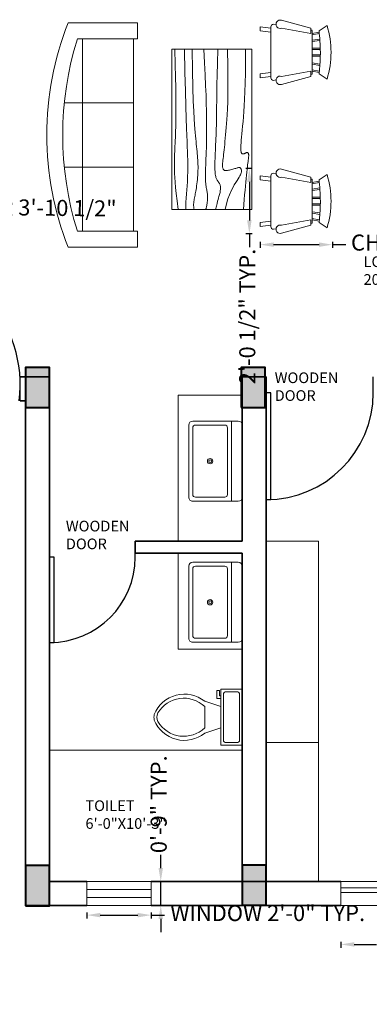
# Model space of a CAD drawing. Units: inches. Extents: x 2845 to 3575, y 808 to 1996.
# Tile 3 of 6: x 3173 to 3304, y 1215 to 1584. Entities that reach past the tile are written whole.
import ezdxf

# ---------------------------------------------------------------- set-up
doc = ezdxf.new("R2010")
doc.units = ezdxf.units.IN
for name, color, linetype, lineweight in [('A-ANNO-DIMS', 2, 'Continuous', 18), ('A-ANNO-TEXT', 7, 'Continuous', 18), ('A-AREA-IDEN', 7, 'Continuous', 18), ('A-COLS', 7, 'Continuous', 40), ('A-DOOR', 34, 'Continuous', 25), ('A-FLOR-CASE', 30, 'Continuous', 18), ('A-FLOR-FIXT', 8, 'Continuous', 18), ('A-FURN', 30, 'Continuous', 18), ('A-GLAZ', 4, 'Continuous', 18), ('A-WALL', 1, 'Continuous', 35)]:
    doc.layers.add(name, color=color, linetype=linetype, lineweight=lineweight)
doc.styles.get("Standard").update_dxf_attribs({"font": 'arial.ttf'})
doc.dimstyles.new('ISO-25', dxfattribs={"dimtxt": 6, "dimasz": 5, "dimexe": 1.25, "dimexo": 0.625, "dimtad": 0, "dimlunit": 4, "dimtxsty": 'Standard', "dimcen": 2.5, "dimclrd": 1, "dimclre": 1, "dimclrt": 1, "dimadec": 0, "dimazin": 0, "dimtfac": 1, "dimtmove": 0, "dimatfit": 3, "dimfxl": 1, "dimfxlon": 1, "dimfrac": 1, "dimarcsym": 0})

# ---------------------------------------------------------------- blocks, each defined once
blk = doc.blocks.new('*U4')
for p, q in [((0, 0), (0, 6)), ((32, 0), (32, 6))]:
    blk.add_line(p, q)
blk.add_lwpolyline([(0, 0), (0, -32), (1.75, -32), (1.75, 0)], close=True)
blk.add_arc((0, 0), 32, 270, 0)
blk = doc.blocks.new('*U5')
for p, q in [((0, 0), (0, 6)), ((40, 0), (40, 6))]:
    blk.add_line(p, q)
blk.add_lwpolyline([(0, 0), (0, -40), (1.75, -40), (1.75, 0)], close=True)
blk.add_arc((0, 0), 40, 270, 0)
blk = doc.blocks.new('Sofa - Roundback 7 ft.')
for p, q in [((-12.00002, -32.4421), (-12.00003, -6.5971)), ((11.99997, -32.4421), (11.99998, -6.5971)), ((-36.000027, -34), (-36.000027, -11.4696)), ((-35.999844, -13.3819), (35.9998, -13.3819)), ((35.99998, -34), (35.99998, -11.4696)), ((-36.000027, -32.4421), (35.99998, -32.4421))]:
    blk.add_line(p, q)
for points in [[(-36.000027, -34), (-42.000027, -34), (-42.000027, -8)], [(41.99998, -8), (41.99998, -34), (35.99998, -34)]]:
    blk.add_lwpolyline(points)
for centre, radius, start, end in [((0, -114.25), 114.25, 68.43141, 111.5686), ((-0.00001, -127.1968), 121.1968, 72.72033, 107.2797)]:
    blk.add_arc(centre, radius, start, end)
blk = doc.blocks.new('Chair - Rocking')
for p, q in [((-8, -4.5), (-10, -1.5)), ((8, -4.5), (10, -1.5)), ((-8.23428, -6.99939), (-8.3093, -7.47958)), ((-8.23041, -7), (8.23915, -7)), ((-7.5, -4.5), (-7, -7)), ((-6.5, -7), (-7.02225, -4.43)), ((-4.5, -7), (-4.96674, -4.19951)), ((-4, -7), (-4.40532, -4.16272)), ((-1.5, -4.05012), (-1.5, -7)), ((-1, -7), (-1, -4.05012)), ((1, -7), (1, -4.04655)), ((1.5, -4.05012), (1.5, -7)), ((4, -7), (4.40187, -4.18694)), ((4.5, -7), (4.96761, -4.19437)), ((6.5, -7), (7, -4.4057)), ((7.5, -4.5), (7, -7)), ((8.31071, -7.48854), (8.23449, -7.00073)), ((-9, -7.5), (-12, -18.49999)), ((-7, -7.5), (-9, -7.5)), ((-9, -18.49999), (-7, -7.5)), ((7, -7.5), (9, -7.5)), ((9, -18.49999), (7, -7.5)), ((9, -7.5), (12, -18.49999)), ((-10.36644, -20.64523), (-10.5, -21.49999)), ((10.5, -21.49999), (10.3575, -20.58798)), ((-9, -22.49999), (-9.5, -26.49999)), ((0, -22.49999), (-9.5, -22.49999)), ((-8, -26.49999), (-7.5, -22.49999)), ((0, -22.49999), (9.5, -22.49999)), ((8, -26.49999), (7.5, -22.49999)), ((9, -22.49999), (9.5, -26.49999)), ((-9.5, -26.49999), (-8, -26.49999)), ((9.5, -26.49999), (8, -26.49999))]:
    blk.add_line(p, q)
for centre, radius, start, end in [((0, -34.08333), 34.08333, 72.93847, 107.0615), ((0, -68.25004), 64.25, 93.92211, 97.15267), ((0, -68.25004), 64.25, 82.84733, 93.92211), ((-10.5, -18.99999), 1.58114, 161.5651, 18.43495), ((-9.5, -21.49999), 1, 180, 270), ((10.5, -18.99999), 1.58114, 161.5651, 18.43495), ((9.5, -21.49999), 1, 270, 0)]:
    blk.add_arc(centre, radius, start, end)
blk = doc.blocks.new('Sink-single - 30 in top')
blk.add_line((-15, -3.999996), (15, -3.999996))
for points in [[(-13.5, 0), (13.5, 0)], [(-15, -18.499996), (-15, -1.5)], [(15, -1.5), (15, -18.499996)], [(-13.5, -17.499996), (-13.5, -6.499996)], [(-12.5, -5.499996), (12.5, -5.499996)], [(13.5, -6.499996), (13.5, -17.499996)], [(13.5, -19.999996), (-13.5, -19.999996)], [(12.5, -18.499996), (-12.5, -18.499996)]]:
    blk.add_lwpolyline(points)
for radius in [1, 0.5]:
    blk.add_circle((0, -11.999996), radius)
for centre, radius, start, end in [((-13.5, -1.5), 1.5, 90, 180), ((13.5, -1.5), 1.5, 0, 90), ((-12.5, -6.499996), 1, 90, 180), ((12.5, -6.499996), 1, 0, 90), ((-12.5, -17.499996), 1, 180, 270), ((12.5, -17.499996), 1, 270, 0), ((-13.5, -18.499996), 1.5, 180, 270), ((13.5, -18.499996), 1.5, 270, 0)]:
    blk.add_arc(centre, radius, start, end)
blk = doc.blocks.new('Toilet - top')
for p, q in [((9.5, -6), (9.5, -2)), ((-10, -8.5), (-8, -8.5)), ((-10, -9.5), (-10, -8.5)), ((-7, -9.5), (-10, -9.5)), ((-8, -8.5), (-8, -8)), ((-7, -8), (-7, -9.5)), ((-4, -8), (-6, -14)), ((4, -8), (6, -14)), ((4, -14), (-4, -14))]:
    blk.add_line(p, q)
blk.add_lwpolyline([(10.5, -8), (10.5, 0), (-10.5, 0), (-10.5, -8)], close=True)
for points in [[(-9.5, -2), (-9.5, -6)], [(8.5, -1), (-8.5, -1)], [(-8.5, -7), (8.5, -7)]]:
    blk.add_lwpolyline(points)
for centre, radius, start, end in [((-8.62, -1.88), 0.884, 81.8699, 188.1301), ((8.62, -1.88), 0.884, 351.8699, 98.1301), ((-8.62, -6.12), 0.884, 171.8699, 278.1301), ((8.62, -6.12), 0.884, 261.8699, 8.1301), ((3.52, -21.58), 12.17, 141.4691, 247.9714), ((4.2, -21.82), 11.33, 136.3677, 238.9468), ((-3.52, -21.58), 12.17, 292.0284, 38.5307), ((-4.2, -21.82), 11.33, 301.053, 43.6321), ((0, -27.88), 4, 245.7318, 294.2682), ((0, -29), 4, 254.8605, 285.1395)]:
    blk.add_arc(centre, radius, start, end)
blk = doc.blocks.new('Table - Rectangular Woodgrain 60 x 30 in.')
for p, q in [((0, 0), (0, -30)), ((60, 0), (0, 0)), ((60, -30), (60, 0)), ((0, -30), (60, -30))]:
    blk.add_line(p, q)
for points in [[(0, -2.4), (4.8155, -2.418), (9.0302, -2.4688), (12.709, -2.5477), (15.9167, -2.65), (18.7181, -2.7711), (21.1781, -2.9063), (23.3616, -3.0508), (25.3333, -3.2), (27.1477, -3.3495), (28.8172, -3.4958), (30.3437, -3.636), (31.7291, -3.7667), (32.9756, -3.8849), (34.0849, -3.9875), (35.059, -4.0714), (35.9, -4.1334), (36.6114, -4.1711), (37.2041, -4.1854), (37.6906, -4.1779), (38.0833, -4.15), (38.3948, -4.1034), (38.6375, -4.0396), (38.8239, -3.9602), (38.9666, -3.8667), (39.0764, -3.7608), (39.1573, -3.6448), (39.2116, -3.521), (39.2416, -3.3917), (39.2498, -3.2593), (39.2385, -3.1261), (39.21, -2.9944), (39.1666, -2.8667), (39.111, -2.7447), (39.0468, -2.6281), (38.978, -2.5163), (38.9083, -2.4083), (38.8418, -2.3035), (38.7823, -2.201), (38.7337, -2.1001), (38.7, -2), (38.6844, -1.9003), (38.6875, -1.8021), (38.7094, -1.707), (38.75, -1.6167), (38.8094, -1.5326), (38.8875, -1.4563), (38.9844, -1.3893), (39.1, -1.3333), (39.2351, -1.2896), (39.3937, -1.2583), (39.5804, -1.2396), (39.8, -1.2333), (40.057, -1.2396), (40.3562, -1.2583), (40.7023, -1.2896), (41.1, -1.3333), (41.5547, -1.3895), (42.0755, -1.4573), (42.6721, -1.5361), (43.3542, -1.625), (44.1316, -1.7233), (45.014, -1.8302), (46.0114, -1.9449), (47.1333, -2.0667), (48.3862, -2.1947), (49.7625, -2.3281), (51.2513, -2.4663), (52.8416, -2.6083), (54.5226, -2.7535), (56.2833, -2.9011), (58.1127, -3.0501), (60, -3.2)], [(0, -9.2), (6.5759, -9.0858), (11.9385, -9.0365), (16.2527, -9.0418), (19.6833, -9.0917), (22.3952, -9.1759), (24.5531, -9.2844), (26.322, -9.4069), (27.8666, -9.5333), (29.3241, -9.6553), (30.7203, -9.7719), (32.0532, -9.8837), (33.3208, -9.9917), (34.5213, -10.0965), (35.6526, -10.199), (36.7128, -10.2999), (37.7, -10.4), (38.6129, -10.4996), (39.4531, -10.5969), (40.223, -10.6895), (40.925, -10.775), (41.5613, -10.8512), (42.1344, -10.9156), (42.6465, -10.966), (43.1, -11), (43.4976, -11.0158), (43.8437, -11.0136), (44.143, -10.9942), (44.4, -10.9583), (44.6195, -10.9069), (44.8062, -10.8406), (44.9648, -10.7603), (45.1, -10.6667), (45.2155, -10.5598), (45.3114, -10.4365), (45.3871, -10.2929), (45.4416, -10.125), (45.4743, -9.929), (45.4844, -9.7011), (45.4709, -9.4371), (45.4333, -9.1333), (45.3716, -8.7883), (45.2896, -8.4104), (45.1919, -8.0107), (45.0833, -7.6), (44.9685, -7.1893), (44.8521, -6.7896), (44.7388, -6.4117), (44.6333, -6.0667), (44.54, -5.7628), (44.4614, -5.4979), (44.4001, -5.2675), (44.3583, -5.0667), (44.3384, -4.8909), (44.3427, -4.7354), (44.3736, -4.5956), (44.4333, -4.4667), (44.5236, -4.3453), (44.6427, -4.2333), (44.7884, -4.1339), (44.9583, -4.05), (45.1501, -3.9849), (45.3614, -3.9417), (45.59, -3.9234), (45.8333, -3.9333), (46.0915, -3.9749), (46.3734, -4.0531), (46.6906, -4.1736), (47.0542, -4.3417), (47.4756, -4.5629), (47.9661, -4.8427), (48.5372, -5.1866), (49.2, -5.6), (49.9676, -6.0844), (50.8594, -6.625), (51.8965, -7.2031), (53.1, -7.8), (54.491, -8.3969), (56.0906, -8.975), (57.9199, -9.5156), (60, -10)], [(0, -12.8), (5.1847, -12.9322), (9.6213, -13.0323), (13.3963, -13.1059), (16.5958, -13.1583), (19.3063, -13.1952), (21.614, -13.2219), (23.6054, -13.2439), (25.3666, -13.2667), (26.9728, -13.2947), (28.4531, -13.3281), (29.8256, -13.3663), (31.1083, -13.4083), (32.3191, -13.4535), (33.476, -13.501), (34.597, -13.5501), (35.7, -13.6), (36.7984, -13.6497), (37.8875, -13.6979), (38.9578, -13.743), (40, -13.7833), (41.0047, -13.8174), (41.9625, -13.8438), (42.864, -13.8607), (43.7, -13.8667), (44.4631, -13.8604), (45.1552, -13.8417), (45.7801, -13.8104), (46.3416, -13.7667), (46.8439, -13.7104), (47.2906, -13.6417), (47.6858, -13.5604), (48.0333, -13.4667), (48.3375, -13.3608), (48.6042, -13.2448), (48.8396, -13.121), (49.05, -12.9917), (49.2417, -12.8593), (49.4208, -12.7261), (49.5937, -12.5944), (49.7667, -12.4667), (49.9452, -12.3451), (50.1323, -12.2313), (50.3303, -12.1268), (50.5416, -12.0333), (50.7686, -11.9524), (51.0135, -11.8854), (51.2788, -11.8341), (51.5666, -11.8), (51.8785, -11.7843), (52.2116, -11.7865), (52.562, -11.8059), (52.926, -11.8417), (53.2998, -11.8931), (53.6795, -11.9594), (54.0614, -12.0397), (54.4416, -12.1333), (54.8223, -12.2401), (55.2293, -12.3625), (55.6942, -12.5037), (56.2489, -12.6667), (56.9251, -12.8547), (57.7545, -13.0708), (58.7689, -13.3182), (60, -13.6)], [(0, -18), (5.124, -17.7273), (9.6609, -17.5057), (13.6705, -17.3303), (17.2125, -17.1958), (20.3467, -17.0973), (23.1328, -17.0297), (25.6307, -16.9878), (27.9, -16.9667), (29.9928, -16.9617), (31.9302, -16.9703), (33.7254, -16.9907), (35.3917, -17.0208), (36.9423, -17.0588), (38.3906, -17.1026), (39.7499, -17.1503), (41.0333, -17.2), (42.2519, -17.2496), (43.4073, -17.2969), (44.4986, -17.3395), (45.525, -17.375), (46.4858, -17.4012), (47.3802, -17.4156), (48.2074, -17.416), (48.9667, -17.4), (49.6583, -17.3662), (50.2872, -17.3167), (50.8595, -17.2547), (51.3812, -17.1833), (51.8584, -17.1057), (52.2971, -17.025), (52.7034, -16.9443), (53.0833, -16.8667), (53.443, -16.7951), (53.789, -16.7313), (54.128, -16.6768), (54.4666, -16.6334), (54.8115, -16.6024), (55.1693, -16.5854), (55.5465, -16.5841), (55.95, -16.6), (56.3828, -16.6337), (56.8346, -16.6823), (57.2915, -16.7418), (57.7396, -16.8084), (58.165, -16.878), (58.5539, -16.9469), (58.8924, -17.0111), (59.1666, -17.0667), (59.3679, -17.1107), (59.5078, -17.1438), (59.6032, -17.1675), (59.6708, -17.1833), (59.7275, -17.193), (59.7901, -17.1979), (59.8753, -17.1998), (60, -17.2)], [(0, -22.4), (8.0098, -22.2501), (14.4094, -22.1011), (19.4168, -21.9535), (23.25, -21.8083), (26.1269, -21.6663), (28.2656, -21.5281), (29.884, -21.3947), (31.2, -21.2667), (32.3967, -21.1448), (33.5172, -21.0292), (34.5697, -20.9198), (35.5625, -20.8167), (36.5037, -20.7198), (37.4015, -20.6292), (38.2642, -20.5448), (39.1, -20.4667), (39.9164, -20.3951), (40.7187, -20.3313), (41.5117, -20.2768), (42.3, -20.2333), (43.0883, -20.2024), (43.8812, -20.1854), (44.6836, -20.1841), (45.5, -20.2), (46.3328, -20.234), (47.1747, -20.2844), (48.0163, -20.3488), (48.8479, -20.425), (49.66, -20.5106), (50.4429, -20.6031), (51.1872, -20.7004), (51.8833, -20.8), (52.5246, -20.8999), (53.1166, -20.9995), (53.6681, -21.0983), (54.1875, -21.1958), (54.6834, -21.2919), (55.1646, -21.3859), (55.6394, -21.4777), (56.1167, -21.5667), (56.6028, -21.6515), (57.0961, -21.7266), (57.5929, -21.7852), (58.0896, -21.8208), (58.5823, -21.8268), (59.0674, -21.7964), (59.5412, -21.723), (60, -21.6)], [(0, -25.2), (8.6355, -25.0504), (15.7026, -24.9031), (21.4049, -24.7606), (25.9458, -24.625), (29.529, -24.4988), (32.3578, -24.3844), (34.6359, -24.284), (36.5667, -24.2), (38.3213, -24.1341), (39.9417, -24.0854), (41.437, -24.0523), (42.8167, -24.0333), (44.0901, -24.0268), (45.2667, -24.0313), (46.3557, -24.0451), (47.3667, -24.0667), (48.309, -24.0947), (49.1928, -24.1287), (50.0284, -24.168), (50.826, -24.2125), (51.5959, -24.2617), (52.3483, -24.3151), (53.0935, -24.3725), (53.8417, -24.4334), (54.6009, -24.497), (55.3699, -24.561), (56.1454, -24.6226), (56.9239, -24.6792), (57.7021, -24.7279), (58.4764, -24.7662), (59.2435, -24.7911), (60, -24.8)], [(0, -28.8), (5.6867, -28.6681), (10.45, -28.5698), (14.407, -28.5012), (17.675, -28.4584), (20.3711, -28.4374), (22.6125, -28.4344), (24.5164, -28.4455), (26.2, -28.4667), (27.762, -28.4947), (29.2276, -28.5281), (30.6033, -28.5663), (31.8958, -28.6084), (33.1118, -28.6535), (34.2578, -28.7011), (35.3405, -28.7501), (36.3666, -28.8), (37.3443, -28.8497), (38.288, -28.8974), (39.2137, -28.9412), (40.1375, -28.9792), (41.0753, -29.0093), (42.0432, -29.0297), (43.0572, -29.0384), (44.1333, -29.0333), (45.2936, -29.0114), (46.5843, -28.9641), (48.0579, -28.8816), (49.7666, -28.7542), (51.7629, -28.5721), (54.0989, -28.3255), (56.8272, -28.0048), (60, -27.6)]]:
    blk.add_lwpolyline(points)
blk = doc.blocks.new('COL-9x15')
h = blk.add_hatch(color=256)
h.dxf.hatch_style = 1
h.paths.add_polyline_path([(0, 0), (9, 0), (9, 15), (0, 15)])
blk.add_lwpolyline([(0, 0), (9, 0), (9, 15), (0, 15)], close=True)
blk = doc.blocks.new('WIN-24')
for p, q in [((0, 9), (0, 0)), ((0, 9), (24, 9)), ((24, 9), (24, 0)), ((0, 6), (24, 6)), ((0, 3), (24, 3)), ((0, 0), (24, 0))]:
    blk.add_line(p, q)
blk = doc.blocks.new('GLAZ-SLIDER-97')
for p, q in [((0, 9), (0, 0)), ((0, 9), (97.12, 9)), ((97.12, 9), (97.12, 0)), ((0, 6.63), (48.56, 6.63)), ((48.56, 4.89), (0, 4.89)), ((48.56, 6.63), (48.56, 4.89)), ((48.56, 2.45), (48.56, 4.19)), ((48.56, 4.19), (97.12, 4.19)), ((0, 0), (97.12, 0)), ((97.12, 2.45), (48.56, 2.45))]:
    blk.add_line(p, q)
blk = doc.blocks.new('*D54')
at = {"layer": 'A-ANNO-DIMS', "color": 1, "lineweight": -2, "transparency": 16777216}
for p, q in [((3094.31, 1514.81), (3094.28, 1512.56)), ((3099.3, 1513.75), (3135.88, 1513.29)), ((3140.89, 1514.23), (3140.86, 1511.98)), ((3140.88, 1513.23), (3145.88, 1513.16))]:
    blk.add_line(p, q, dxfattribs=at)
at = {"layer": 'A-ANNO-DIMS', "color": 1, "transparency": 16777216}
for points in [[(3099.31, 1514.58), (3099.29, 1512.91), (3094.3, 1513.81)], [(3135.89, 1514.12), (3135.87, 1512.45), (3140.88, 1513.23)]]:
    blk.add_solid(points, dxfattribs=at)
at = {"layer": 'Defpoints', "color": 0, "transparency": 16777216}
for p in [(3094.39, 1520.79), (3140.96, 1520.21), (3140.88, 1513.23)]:
    blk.add_point(p, dxfattribs=at)
at = {"layer": 'A-ANNO-DIMS', "color": 1, "transparency": 16777216, "insert": (3177.96, 1512.76), "char_height": 6, "attachment_point": 5, "rotation": 359.2832}
blk.add_mtext('CHAIR 3\'-10 1/2"', dxfattribs=at)
blk = doc.blocks.new('*D56')
at = {"layer": 'A-ANNO-DIMS', "color": 1, "lineweight": -2, "transparency": 16777216}
for p, q in [((3262.84, 1500.65), (3262.84, 1498.4)), ((3267.84, 1499.65), (3284.84, 1499.65)), ((3289.84, 1500.65), (3289.84, 1498.4)), ((3289.84, 1499.65), (3294.84, 1499.65))]:
    blk.add_line(p, q, dxfattribs=at)
at = {"layer": 'A-ANNO-DIMS', "color": 1, "transparency": 16777216}
for points in [[(3267.84, 1500.49), (3267.84, 1498.82), (3262.84, 1499.65)], [(3284.84, 1500.49), (3284.84, 1498.82), (3289.84, 1499.65)]]:
    blk.add_solid(points, dxfattribs=at)
at = {"layer": 'Defpoints', "color": 0, "transparency": 16777216}
for p in [(3262.84, 1503.7), (3289.84, 1503.7), (3289.84, 1499.65)]:
    blk.add_point(p, dxfattribs=at)
at = {"layer": 'A-ANNO-DIMS', "color": 1, "transparency": 16777216, "insert": (3327.92, 1499.65), "char_height": 6, "attachment_point": 5}
blk.add_mtext('CHAIR 2\'-3" TYP.', dxfattribs=at)
blk = doc.blocks.new('*D57')
at = {"layer": 'A-ANNO-DIMS', "color": 1, "lineweight": -2, "transparency": 16777216}
for p, q in [((3259.79, 1528.14), (3257.54, 1528.14)), ((3258.79, 1523.14), (3258.79, 1508.7)), ((3259.79, 1503.7), (3257.54, 1503.7)), ((3258.79, 1503.7), (3258.79, 1498.7))]:
    blk.add_line(p, q, dxfattribs=at)
at = {"layer": 'A-ANNO-DIMS', "color": 1, "transparency": 16777216}
for points in [[(3257.96, 1523.14), (3259.62, 1523.14), (3258.79, 1528.14)], [(3257.96, 1508.7), (3259.62, 1508.7), (3258.79, 1503.7)]]:
    blk.add_solid(points, dxfattribs=at)
at = {"layer": 'Defpoints', "color": 0, "transparency": 16777216}
for p in [(3262.84, 1528.14), (3258.79, 1503.7), (3262.84, 1503.7)]:
    blk.add_point(p, dxfattribs=at)
at = {"layer": 'A-ANNO-DIMS', "color": 1, "transparency": 16777216, "insert": (3258.79, 1472.75), "char_height": 6, "attachment_point": 5, "rotation": 90}
blk.add_mtext('2\'-0 1/2" TYP.', dxfattribs=at)
blk = doc.blocks.new('*D58')
at = {"layer": 'A-ANNO-DIMS', "color": 1, "lineweight": -2, "transparency": 16777216}
for p, q in [((3198.07, 1249.57), (3198.07, 1247.32)), ((3203.07, 1248.57), (3217.07, 1248.57)), ((3222.07, 1249.57), (3222.07, 1247.32)), ((3222.07, 1248.57), (3227.07, 1248.57))]:
    blk.add_line(p, q, dxfattribs=at)
at = {"layer": 'A-ANNO-DIMS', "color": 1, "transparency": 16777216}
for points in [[(3203.07, 1249.41), (3203.07, 1247.74), (3198.07, 1248.57)], [(3217.07, 1249.41), (3217.07, 1247.74), (3222.07, 1248.57)]]:
    blk.add_solid(points, dxfattribs=at)
at = {"layer": 'Defpoints', "color": 0, "transparency": 16777216}
for p in [(3198.07, 1252.17), (3222.07, 1252.17), (3222.07, 1248.57)]:
    blk.add_point(p, dxfattribs=at)
at = {"layer": 'A-ANNO-DIMS', "color": 1, "transparency": 16777216, "insert": (3265.66, 1248.57), "char_height": 6, "attachment_point": 5}
blk.add_mtext('WINDOW 2\'-0" TYP.', dxfattribs=at)
blk = doc.blocks.new('*D59')
at = {"layer": 'A-ANNO-DIMS', "color": 1, "lineweight": -2, "transparency": 16777216}
for p, q in [((3225.67, 1266.17), (3225.67, 1271.17)), ((3224.67, 1261.17), (3226.92, 1261.17)), ((3225.67, 1252.17), (3225.67, 1261.17)), ((3224.67, 1252.17), (3226.92, 1252.17)), ((3225.67, 1247.17), (3225.67, 1242.17))]:
    blk.add_line(p, q, dxfattribs=at)
at = {"layer": 'A-ANNO-DIMS', "color": 1, "transparency": 16777216}
for points in [[(3224.84, 1266.17), (3226.5, 1266.17), (3225.67, 1261.17)], [(3224.84, 1247.17), (3226.5, 1247.17), (3225.67, 1252.17)]]:
    blk.add_solid(points, dxfattribs=at)
at = {"layer": 'Defpoints', "color": 0, "transparency": 16777216}
for p in [(3222.07, 1261.17), (3225.67, 1261.17), (3222.07, 1252.17)]:
    blk.add_point(p, dxfattribs=at)
at = {"layer": 'A-ANNO-DIMS', "color": 1, "transparency": 16777216, "insert": (3225.67, 1290.08), "char_height": 6, "attachment_point": 5, "rotation": 90}
blk.add_mtext('0\'-9" TYP.', dxfattribs=at)
blk = doc.blocks.new('*D64')
at = {"layer": 'A-ANNO-DIMS', "color": 1, "lineweight": -2, "transparency": 16777216}
for p, q in [((3293.03, 1238.6), (3293.03, 1236.35)), ((3298.03, 1237.6), (3306.39, 1237.6)), ((3385.15, 1237.6), (3376.79, 1237.6)), ((3390.15, 1238.6), (3390.15, 1236.35))]:
    blk.add_line(p, q, dxfattribs=at)
at = {"layer": 'A-ANNO-DIMS', "color": 1, "transparency": 16777216}
for points in [[(3298.03, 1238.44), (3298.03, 1236.77), (3293.03, 1237.6)], [(3385.15, 1238.44), (3385.15, 1236.77), (3390.15, 1237.6)]]:
    blk.add_solid(points, dxfattribs=at)
at = {"layer": 'Defpoints', "color": 0, "transparency": 16777216}
for p in [(3293.03, 1252.17), (3390.15, 1252.17), (3390.15, 1237.6)]:
    blk.add_point(p, dxfattribs=at)
at = {"layer": 'A-ANNO-DIMS', "color": 1, "transparency": 16777216, "insert": (3341.59, 1237.6), "char_height": 6, "attachment_point": 5}
blk.add_mtext('SLIDER 8\'-1" TYP.', dxfattribs=at)
blk = doc.blocks.new('*D73')
at = {"layer": 'A-ANNO-DIMS', "color": 1, "lineweight": -2, "transparency": 16777216}
for p, q in [((2986.12, 844.33), (2986.12, 842.08)), ((2991.12, 843.33), (3069.97, 843.33)), ((3170.12, 843.33), (3091.26, 843.33)), ((3175.12, 844.33), (3175.12, 842.08))]:
    blk.add_line(p, q, dxfattribs=at)
at = {"layer": 'A-ANNO-DIMS', "color": 1, "transparency": 16777216}
for points in [[(2991.12, 844.17), (2991.12, 842.5), (2986.12, 843.33)], [(3170.12, 844.17), (3170.12, 842.5), (3175.12, 843.33)]]:
    blk.add_solid(points, dxfattribs=at)
at = {"layer": 'Defpoints', "color": 0, "transparency": 16777216}
for p in [(2986.12, 1250.42), (3175.12, 1252.17), (3175.12, 843.33)]:
    blk.add_point(p, dxfattribs=at)
at = {"layer": 'A-ANNO-DIMS', "color": 1, "transparency": 16777216, "insert": (3080.62, 843.33), "char_height": 6, "attachment_point": 5}
blk.add_mtext('15\'-9"', dxfattribs=at)

msp = doc.modelspace()

# ---------------------------------------------------------------- linework, layer by layer
at = {"layer": 'A-DOOR'}
for p, q in [((3173.116, 1441.173), (3173.116, 1450.173)), ((3216.116, 1388.673), (3216.116, 1384.173))]:
    msp.add_line(p, q, dxfattribs=at)
msp.add_arc((3125.116, 1447.173), 48, 352.81924, 92.38802, dxfattribs=at)
at = {"layer": 'A-FLOR-CASE'}
for p, q in [((3232.116, 1388.673), (3232.116, 1443.342)), ((3256.116, 1443.342), (3232.116, 1443.342)), ((3265.116, 1388.673), (3279.948, 1388.673)), ((3279.948, 1388.673), (3284.68, 1388.673)), ((3284.68, 1388.673), (3284.68, 1261.173)), ((3232.116, 1384.173), (3232.116, 1360.173)), ((3232.116, 1360.173), (3232.116, 1348.173)), ((3232.116, 1348.173), (3256.116, 1348.173)), ((3265.116, 1313.244), (3284.68, 1313.244))]:
    msp.add_line(p, q, dxfattribs=at)
at = {"layer": 'A-FLOR-FIXT'}
msp.add_line((3256.116, 1310.347), (3184.116, 1310.347), dxfattribs=at)
at = {"layer": 'A-WALL'}
for p, q in [((3184.116, 1450.173), (3173.116, 1450.173)), ((3175.116, 1252.173), (3175.116, 1450.173)), ((3175.116, 1450.173), (3175.116, 1441.173)), ((3184.116, 1261.173), (3184.116, 1450.173)), ((3256.116, 1388.673), (3256.116, 1450.173)), ((3265.116, 1450.173), (3256.116, 1450.173)), ((3265.116, 1261.173), (3265.116, 1450.173)), ((3175.116, 1441.173), (3173.116, 1441.173)), ((3175.116, 1441.173), (3173.116, 1441.173)), ((3256.116, 1388.673), (3216.116, 1388.673)), ((3256.116, 1384.173), (3216.116, 1384.173)), ((3256.116, 1261.173), (3256.116, 1384.173)), ((3198.07, 1261.173), (3184.116, 1261.173)), ((3256.116, 1261.173), (3222.07, 1261.173)), ((3293.028, 1261.173), (3256.116, 1261.173)), ((3198.07, 1252.173), (3175.116, 1252.173)), ((3293.028, 1252.173), (3222.07, 1252.173))]:
    msp.add_line(p, q, dxfattribs=at)

# ---------------------------------------------------------------- block references
at = {"layer": 'A-COLS'}
for p in [(3175.116, 1438.625), (3255.744, 1438.625), (3175.116, 1252.102), (3256.116, 1252.239)]:
    msp.add_blockref('COL-9x15', p, dxfattribs=at)
at = {"layer": 'A-DOOR'}
for name, p in [('*U5', (3265.116, 1444.173)), ('*U4', (3184.116, 1382.673))]:
    msp.add_blockref(name, p, dxfattribs=at)
at = {"layer": 'A-FLOR-FIXT', "rotation": 270}
for name, p in [('Sink-single - 30 in top', (3256.116, 1418.579)), ('Sink-single - 30 in top', (3256.116, 1365.745)), ('Toilet - top', (3256.116, 1322.673))]:
    msp.add_blockref(name, p, dxfattribs=at)
at = {"layer": 'A-FURN'}
for name, p, rotation in [('Sofa - Roundback 7 ft.', (3183.018, 1540.702), 90), ('Chair - Rocking', (3289.34, 1571.678), 270), ('Table - Rectangular Woodgrain 60 x 30 in.', (3259.781, 1572.858), 270), ('Chair - Rocking', (3289.34, 1515.92), 270)]:
    msp.add_blockref(name, p, dxfattribs=dict(at, rotation=rotation))
at = {"layer": 'A-GLAZ'}
for name, p in [('WIN-24', (3198.07, 1252.173)), ('GLAZ-SLIDER-97', (3293.028, 1252.173))]:
    msp.add_blockref(name, p, dxfattribs=at)

# ---------------------------------------------------------------- texts
at = {"layer": 'A-ANNO-TEXT', "char_height": 4, "attachment_point": 1}
for width, insert in [(35.3288, (3268.271, 1451.807)), (39.54771, (3190.182, 1396.261))]:
    msp.add_mtext_dynamic_manual_height_columns('WOODEN DOOR', width=width, gutter_width=12.5, heights=[0], dxfattribs=dict(at, insert=insert))
at = {"layer": 'A-AREA-IDEN', "char_height": 4, "attachment_point": 1}
for s, insert in [('LOBBY\\P20\'-0"X14\'-6"', (3301.502, 1495.272)), ('TOILET\\P6\'-0"X10\'-3"', (3197.503, 1291.55))]:
    msp.add_mtext_dynamic_manual_height_columns(s, width=45.255, gutter_width=12.5, heights=[0], dxfattribs=dict(at, insert=insert))

# ---------------------------------------------------------------- dimensions: what is measured, and where the dimension line sits
at = {"layer": 'A-ANNO-DIMS'}
for base, p1, p2, angle, text, picture, middle in [((3140.876, 1513.225), (3094.387, 1520.795), (3140.963, 1520.212), 359.28319, 'CHAIR <>', '*D54', (3177.963, 1512.761)), ((3258.79, 1503.702), (3262.84, 1528.137), (3262.84, 1503.702), 270, '<> TYP.', '*D57', (3258.79, 1472.749)), ((3225.67, 1261.173), (3222.07, 1252.173), (3222.07, 1261.173), 90, '<> TYP.', '*D59', (3225.67, 1290.084))]:
    dim = msp.add_linear_dim(base=base, p1=p1, p2=p2, angle=angle, text=text, dimstyle='ISO-25', override={"dimdec": 1, "dimlfac": 1, "dimrnd": 0, "dimzin": 1, "dimdsep": 46, "dimlunit": 4, "dimfrac": 2}, dxfattribs=at)
    dim.commit()
    dim.dimension.update_dxf_attribs({"geometry": picture, "text_midpoint": middle})
for base, p1, p2, text, picture, middle in [((3289.84, 1499.652), (3262.84, 1503.702), (3289.84, 1503.702), 'CHAIR <> TYP.', '*D56', (3327.92, 1499.652)), ((3222.07, 1248.573), (3198.07, 1252.173), (3222.07, 1252.173), 'WINDOW <> TYP.', '*D58', (3265.657, 1248.573)), ((3390.151, 1237.604), (3293.028, 1252.173), (3390.151, 1252.173), 'SLIDER <> TYP.', '*D64', (3341.59, 1237.604))]:
    dim = msp.add_linear_dim(base=base, p1=p1, p2=p2, text=text, dimstyle='ISO-25', override={"dimdec": 1, "dimlfac": 1, "dimrnd": 0, "dimzin": 1, "dimdsep": 46, "dimlunit": 4, "dimfrac": 2}, dxfattribs=at)
    dim.commit()
    dim.dimension.update_dxf_attribs({"geometry": picture, "text_midpoint": middle})
dim = msp.add_linear_dim(base=(3175.116, 843.335), p1=(2986.116, 1250.417), p2=(3175.116, 1252.173), dimstyle='ISO-25', override={"dimdec": 1, "dimlfac": 1, "dimrnd": 0, "dimzin": 1, "dimdsep": 46, "dimlunit": 4, "dimfrac": 2}, dxfattribs=at)
dim.commit()
dim.dimension.update_dxf_attribs({"geometry": '*D73', "text_midpoint": (3080.616, 843.335)})

doc.saveas('drawing.dxf')
